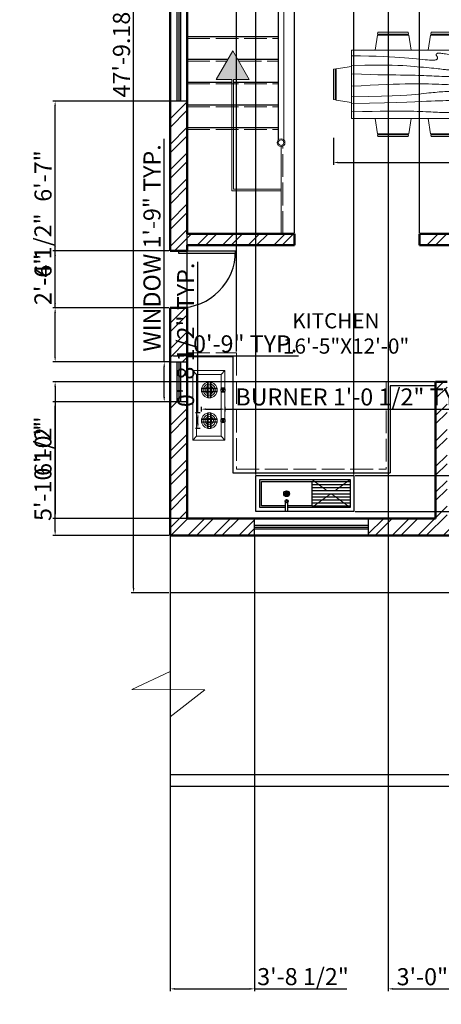
# Model space of a CAD drawing. Units: inches. Extents: x 635 to 1184, y 1837 to 2697.
# Tile 1 of 6: x 635 to 857, y 1837 to 2356. Entities that reach past the tile are written whole.
import ezdxf

# ---------------------------------------------------------------- set-up
doc = ezdxf.new("R2010")
doc.units = ezdxf.units.IN
doc.linetypes.add('ACAD_ISO02W100', pattern=[15, 12, -3])
for name, color, linetype, lineweight in [('A-ANNO-DIMS', 2, 'Continuous', 18), ('A-ANNO-SYMB', 7, 'Continuous', 18), ('A-AREA-IDEN', 7, 'Continuous', 25), ('A-CSWK', 8, 'Continuous', 25), ('A-CSWK-HIDN', 8, 'ACAD_ISO02W100', 13), ('A-DOOR', 4, 'Continuous', 25), ('A-EQPM', 9, 'Continuous', 18), ('A-FLOR-FIXT', 8, 'Continuous', 25), ('A-FLOR-FIXT-HIDN', 8, 'ACAD_ISO02W100', 13), ('A-FLOR-RAIL', 7, 'Continuous', 18), ('A-FLOR-RAIL-HIDN', 8, 'ACAD_ISO02W100', 13), ('A-FLOR-STRS', 7, 'Continuous', 25), ('A-FLOR-STRS-HIDN', 8, 'ACAD_ISO02W100', 13), ('A-FURN', 8, 'Continuous', 18), ('A-GLAZ', 244, 'Continuous', 25), ('A-WALL', 7, 'Continuous', 50), ('A-WALL-PATT', 252, 'Continuous', 13), ('C-ROAD', 8, 'Continuous', 25)]:
    doc.layers.add(name, color=color, linetype=linetype, lineweight=lineweight)
doc.styles.get("Standard").update_dxf_attribs({"font": 'arial.ttf'})
doc.dimstyles.new('ISO-25', dxfattribs={"dimtxt": 9, "dimasz": 2.5, "dimexe": 1.25, "dimexo": 0.625, "dimtad": 1, "dimlunit": 3, "dimtxsty": 'Standard', "dimcen": 2.5, "dimadec": 0, "dimazin": 0, "dimtfac": 1, "dimtmove": 0, "dimatfit": 3, "dimfxl": 1, "dimarcsym": 0})

# ---------------------------------------------------------------- blocks, each defined once
blk = doc.blocks.new('*U5')
for p, q in [((-40, 0), (-40, 6)), ((0, 0), (0, 6))]:
    blk.add_line(p, q)
blk.add_lwpolyline([(0, 0), (0, -40), (-1.75, -40), (-1.75, 0)], close=True)
blk.add_arc((0, 0), 40, 180, 270)
blk = doc.blocks.new('Dining Set - 36 x 72 in.')
for p, q in [((-22.2343, 26.00059), (-23.4847, 17.99762)), ((-22.2304, 26), (-5.7608, 26)), ((-22, 27.5), (-22.1562, 26.50042)), ((-5.8416, 26.5), (-22.1534, 26.5)), ((-22, 27.5), (-6, 27.5)), ((-5.8437, 26.49966), (-6, 27.5)), ((-4.5152, 17.99762), (-5.7655, 25.99926)), ((5.7657, 26.00059), (4.5153, 17.99762)), ((5.7696, 26), (22.2392, 26)), ((6, 27.5), (5.8438, 26.50042)), ((22.1584, 26.5), (5.8466, 26.5)), ((6, 27.5), (22, 27.5)), ((22.1563, 26.49966), (22, 27.5)), ((23.4848, 17.99762), (22.2345, 25.99926)), ((36, 18), (-36, 18)), ((-36, 18), (-36, -18)), ((36, -18), (36, 18)), ((-45.5, 8), (-44.5004, 8.15617)), ((-45.5, 8), (-45.5, -8)), ((-44.5, -8.15843), (-44.5, 8.15338)), ((-44.0006, 8.23428), (-35.9976, 9.48474)), ((-44, 8.23041), (-44, -8.23915)), ((44.0006, 8.23428), (35.9976, 9.48474)), ((44, 8.23041), (44, -8.23915)), ((44.5, -8.15843), (44.5, 8.15338)), ((45.5, 8), (44.5005, 8.15617)), ((45.5, 8), (45.5, -8)), ((-44.4997, -8.15631), (-45.5, -8)), ((-35.9976, -9.48476), (-43.9993, -8.2345)), ((35.9976, -9.48476), (43.9993, -8.2345)), ((44.4997, -8.15631), (45.5, -8)), ((-36, -18), (36, -18)), ((-22.2343, -26.0006), (-23.4847, -17.99762)), ((-4.5152, -17.99762), (-5.7655, -25.99928)), ((5.7657, -26.0006), (4.5153, -17.99762)), ((23.4848, -17.99762), (22.2345, -25.99928)), ((-22.2304, -26), (-5.7608, -26)), ((-22, -27.5), (-22.1562, -26.50044)), ((-5.8416, -26.5), (-22.1534, -26.5)), ((-22, -27.5), (-6, -27.5)), ((-5.8437, -26.49967), (-6, -27.5)), ((5.7696, -26), (22.2392, -26)), ((6, -27.5), (5.8438, -26.50044)), ((22.1584, -26.5), (5.8466, -26.5)), ((6, -27.5), (22, -27.5)), ((22.1563, -26.49967), (22, -27.5))]:
    blk.add_line(p, q)
for points in [[(-36, 15), (-31.1772, 14.97754), (-26.8079, 14.91406), (-22.8538, 14.81543), (-19.276, 14.6875), (-16.0362, 14.53613), (-13.0957, 14.36718), (-10.4159, 14.18652), (-7.9583, 14), (-5.6904, 13.81315), (-3.6035, 13.63021), (-1.6954, 13.45508), (0.0365, 13.29166), (1.5945, 13.14388), (2.9811, 13.01562), (4.1988, 12.9108), (5.25, 12.83333), (6.1393, 12.78613), (6.8802, 12.76823), (7.4883, 12.77767), (7.9792, 12.8125), (8.3685, 12.87077), (8.6719, 12.95052), (8.9049, 13.0498), (9.0833, 13.16666), (9.2205, 13.29899), (9.3216, 13.44401), (9.3895, 13.59879), (9.4271, 13.76041), (9.4373, 13.92594), (9.4232, 14.09245), (9.3875, 14.257), (9.3333, 14.41666), (9.2638, 14.56917), (9.1836, 14.71484), (9.0975, 14.85465), (9.0104, 14.98958), (8.9272, 15.1206), (8.8529, 15.2487), (8.7922, 15.37483), (8.75, 15.5), (8.7305, 15.62467), (8.7344, 15.74739), (8.7617, 15.86621), (8.8125, 15.97916), (8.8867, 16.08431), (8.9844, 16.17968), (9.1055, 16.26334), (9.25, 16.33333), (9.4189, 16.38802), (9.6172, 16.42708), (9.8506, 16.45052), (10.125, 16.45833), (10.4463, 16.45052), (10.8203, 16.42708), (11.2529, 16.38802), (11.75, 16.33333), (12.3184, 16.26318), (12.9694, 16.17838), (13.7151, 16.07991), (14.5677, 15.96875), (15.5395, 15.84586), (16.6426, 15.71224), (17.8893, 15.56884), (19.2917, 15.41666), (20.859, 15.25667), (22.5879, 15.08984), (24.4721, 14.91715), (26.5052, 14.73958), (28.6809, 14.5581), (30.9929, 14.3737), (33.4347, 14.18733), (36, 14)], [(-36, 10), (-28.9766, 10.14274), (-23.1725, 10.20442), (-18.4241, 10.19775), (-14.5677, 10.13541), (-11.4399, 10.03011), (-8.877, 9.89453), (-6.7154, 9.74137), (-4.7917, 9.58333), (-2.9698, 9.43082), (-1.2246, 9.28515), (0.4415, 9.14534), (2.026, 9.01041), (3.5266, 8.87939), (4.9408, 8.7513), (6.266, 8.62516), (7.5, 8.5), (8.6411, 8.37549), (9.6914, 8.2539), (10.6538, 8.13818), (11.5312, 8.03125), (12.3267, 7.93603), (13.043, 7.85547), (13.6831, 7.79248), (14.25, 7.75), (14.7471, 7.7303), (15.1797, 7.73307), (15.5537, 7.75732), (15.875, 7.80208), (16.1494, 7.86637), (16.3828, 7.94922), (16.5811, 8.04964), (16.75, 8.16666), (16.8944, 8.29915), (17.0143, 8.44531), (17.1089, 8.60319), (17.1771, 8.77083), (17.218, 8.94629), (17.2305, 9.1276), (17.2137, 9.31282), (17.1667, 9.5), (17.0895, 9.6875), (16.987, 9.875), (16.8649, 10.0625), (16.7292, 10.25), (16.5856, 10.4375), (16.4401, 10.625), (16.2985, 10.8125), (16.1667, 11), (16.05, 11.18733), (15.9518, 11.3737), (15.8752, 11.5581), (15.8229, 11.73958), (15.798, 11.91715), (15.8034, 12.08984), (15.842, 12.25667), (15.9167, 12.41666), (16.0295, 12.56836), (16.1784, 12.70833), (16.3605, 12.83268), (16.5729, 12.9375), (16.8127, 13.01888), (17.0768, 13.07291), (17.3625, 13.0957), (17.6667, 13.08333), (17.9894, 13.03312), (18.3418, 12.94726), (18.7382, 12.82918), (19.1927, 12.68229), (19.7195, 12.51001), (20.3327, 12.31575), (21.0465, 12.10294), (21.875, 11.875), (22.8357, 11.63354), (23.959, 11.37304), (25.2786, 11.08618), (26.8282, 10.76562), (28.6414, 10.40405), (30.752, 9.99414), (33.1936, 9.52856), (36, 9)], [(-36, 5.5), (-30.7157, 5.3348), (-26.069, 5.20963), (-21.9946, 5.11767), (-18.4271, 5.05208), (-15.3009, 5.00602), (-12.5508, 4.97265), (-10.1112, 4.94515), (-7.9167, 4.91666), (-5.909, 4.88167), (-4.0586, 4.83984), (-2.3429, 4.79215), (-0.7396, 4.73958), (0.7739, 4.6831), (2.22, 4.6237), (3.6213, 4.56233), (5, 4.5), (6.373, 4.43782), (7.7344, 4.3776), (9.0723, 4.32129), (10.375, 4.27083), (11.6309, 4.22819), (12.8281, 4.19531), (13.9551, 4.17415), (15, 4.16666), (15.954, 4.17448), (16.819, 4.19791), (17.6001, 4.23698), (18.3021, 4.29166), (18.9299, 4.36198), (19.4883, 4.44791), (19.9823, 4.54948), (20.4167, 4.66666), (20.7969, 4.79899), (21.1302, 4.94401), (21.4245, 5.09879), (21.6875, 5.26041), (21.9271, 5.42594), (22.1511, 5.59245), (22.3672, 5.757), (22.5834, 5.91666), (22.8065, 6.06868), (23.0404, 6.21093), (23.2879, 6.34147), (23.5521, 6.45833), (23.8358, 6.55957), (24.142, 6.64323), (24.4735, 6.70735), (24.8334, 6.75), (25.2235, 6.76969), (25.642, 6.76692), (26.0858, 6.74267), (26.5521, 6.69791), (27.0379, 6.63362), (27.5404, 6.55078), (28.0565, 6.45036), (28.5834, 6.33333), (29.1242, 6.19987), (29.7071, 6.04687), (30.3661, 5.87044), (31.1354, 5.66666), (32.0493, 5.43164), (33.142, 5.16146), (34.4475, 4.85221), (36, 4.5)], [(-36, -1), (-30.7915, -0.6591), (-26.0195, -0.38216), (-21.6519, -0.16284), (-17.6563, 0.00521), (-14.0005, 0.12833), (-10.6523, 0.21289), (-7.5796, 0.26522), (-4.75, 0.29166), (-2.134, 0.29793), (0.2878, 0.28711), (2.5317, 0.26163), (4.6146, 0.22396), (6.5529, 0.17651), (8.3633, 0.12174), (10.0623, 0.06209), (11.6667, 0), (13.1899, -0.06201), (14.6341, -0.1211), (15.9982, -0.17432), (17.2813, -0.21875), (18.4823, -0.25147), (19.6003, -0.26953), (20.6343, -0.27002), (21.5834, -0.25), (22.4481, -0.20768), (23.2357, -0.14584), (23.9549, -0.06836), (24.6146, 0.02083), (25.2235, 0.11784), (25.7904, 0.21875), (26.3241, 0.31966), (26.8334, 0.41666), (27.3265, 0.50618), (27.8099, 0.58593), (28.2894, 0.65397), (28.7709, 0.70833), (29.2601, 0.74707), (29.763, 0.76823), (30.2855, 0.76985), (30.8334, 0.75), (31.4088, 0.70784), (31.9994, 0.64713), (32.589, 0.57275), (33.1615, 0.48958), (33.7008, 0.4025), (34.1908, 0.3164), (34.6153, 0.23616), (34.9584, 0.16666), (35.2099, 0.11165), (35.3848, 0.07031), (35.504, 0.04069), (35.5886, 0.02083), (35.6594, 0.00879), (35.7377, 0.0026), (35.8442, 0.00032), (36, 0)], [(-36, -6.5), (-27.1843, -6.31267), (-20.084, -6.1263), (-14.469, -5.9419), (-10.1094, -5.76042), (-6.7752, -5.58285), (-4.2363, -5.41016), (-2.2629, -5.24333), (-0.625, -5.08334), (0.8708, -4.93099), (2.2715, -4.78646), (3.5872, -4.64974), (4.8281, -4.52084), (6.0046, -4.39974), (7.127, -4.28646), (8.2053, -4.18099), (9.25, -4.08334), (10.2705, -3.99382), (11.2734, -3.91407), (12.2647, -3.84603), (13.25, -3.79167), (14.2354, -3.75293), (15.2266, -3.73177), (16.2295, -3.73015), (17.25, -3.75), (18.2912, -3.79248), (19.3451, -3.85547), (20.4009, -3.93604), (21.4479, -4.03125), (22.4754, -4.13819), (23.4727, -4.25391), (24.4289, -4.37549), (25.3334, -4.5), (26.1785, -4.62492), (26.9694, -4.74935), (27.7145, -4.87281), (28.4219, -4.99479), (29.1, -5.11483), (29.7572, -5.23242), (30.4016, -5.34709), (31.0417, -5.45834), (31.6837, -5.56437), (32.3262, -5.65821), (32.9658, -5.73153), (33.599, -5.77604), (34.2224, -5.78345), (34.8327, -5.74545), (35.4264, -5.65373), (36, -5.5)], [(-36, -10), (-26.4022, -9.81299), (-18.4675, -9.62891), (-11.9839, -9.45069), (-6.7396, -9.28125), (-2.5226, -9.12354), (0.8789, -8.98047), (3.6769, -8.85498), (6.0833, -8.75), (8.2767, -8.66765), (10.3021, -8.60677), (12.1712, -8.56543), (13.8958, -8.54167), (15.4876, -8.53353), (16.9583, -8.53907), (18.3197, -8.55632), (19.5834, -8.58334), (20.7616, -8.61841), (21.8685, -8.66081), (22.9188, -8.71004), (23.9271, -8.76563), (24.9081, -8.82707), (25.8763, -8.89388), (26.8465, -8.96558), (27.8334, -9.04167), (28.8474, -9.12118), (29.8828, -9.20117), (30.93, -9.27824), (31.9792, -9.34896), (33.0205, -9.40991), (34.0443, -9.45768), (35.0407, -9.48885), (36, -9.5)], [(-36, -14.5), (-30.0881, -14.33513), (-25.0332, -14.21224), (-20.7312, -14.12647), (-17.0781, -14.07292), (-13.97, -14.04671), (-11.3027, -14.04297), (-8.9724, -14.05681), (-6.875, -14.08334), (-4.9224, -14.11833), (-3.0905, -14.16016), (-1.3709, -14.20785), (0.2448, -14.26042), (1.7647, -14.3169), (3.1973, -14.3763), (4.5507, -14.43767), (5.8333, -14.5), (7.0554, -14.5621), (8.235, -14.62175), (9.3922, -14.67652), (10.5469, -14.72396), (11.7192, -14.76164), (12.929, -14.78711), (14.1965, -14.79794), (15.5417, -14.79167), (16.9933, -14.76424), (18.6152, -14.70508), (20.4804, -14.60197), (22.6615, -14.44271), (25.2312, -14.21509), (28.2624, -13.9069), (31.8277, -13.50594), (36, -13)]]:
    blk.add_lwpolyline(points)
blk = doc.blocks.new('*D17')
at = {"layer": 'A-ANNO-DIMS', "color": 0, "lineweight": -2, "transparency": 16777216}
for p, q in [((713.66, 2627.14), (693.72, 2627.14)), ((694.97, 2056.46), (694.97, 2624.64)), ((713.66, 2053.96), (693.72, 2053.96))]:
    blk.add_line(p, q, dxfattribs=at)
at = {"layer": 'A-ANNO-DIMS', "color": 0, "transparency": 16777216}
for points in [[(694.56, 2624.64), (695.39, 2624.64), (694.97, 2627.14)], [(694.56, 2056.46), (695.39, 2056.46), (694.97, 2053.96)]]:
    blk.add_solid(points, dxfattribs=at)
at = {"layer": 'DEFPOINTS', "color": 0, "transparency": 16777216}
for p in [(694.97, 2627.14), (714.28, 2627.14), (714.28, 2053.96)]:
    blk.add_point(p, dxfattribs=at)
at = {"layer": 'A-ANNO-DIMS', "color": 0, "transparency": 16777216, "insert": (689.75, 2340.55), "char_height": 9, "attachment_point": 5, "rotation": 90}
blk.add_mtext('47\'-9.18"', dxfattribs=at)
blk = doc.blocks.new('WIN-21IN')
for p, q in [((3.5, 21), (3.5, 0)), ((4.5, 21), (4.5, 0)), ((5.5, 21), (5.5, 0))]:
    blk.add_line(p, q)
blk.add_lwpolyline([(0, 21), (9, 21), (9, 0), (0, 0)], close=True)
blk = doc.blocks.new('WIN-60IN')
for p, q in [((0, 5.5), (60, 5.5)), ((0, 4.5), (60, 4.5)), ((0, 3.5), (60, 3.5))]:
    blk.add_line(p, q)
blk.add_lwpolyline([(0, 9), (60, 9), (60, 0), (0, 0)], close=True)
blk = doc.blocks.new('COOKTOP-BURNER-WITH-CONTROL')
for p, q in [((3.26, 8.21), (3.26, 0.1)), ((3.56, 8.27), (3.56, 5.06)), ((4.76, 8.27), (4.76, 5.06)), ((5.06, 8.21), (5.06, 0.1)), ((11.16, 5.31), (11.16, 3)), ((11.56, 5.31), (11.56, 3)), ((0.04, 4.76), (3.26, 4.76)), ((0.04, 3.56), (3.26, 3.56)), ((0.1, 5.06), (8.21, 5.06)), ((0.1, 3.26), (8.21, 3.26)), ((3.56, 4.76), (3.56, 3.56)), ((3.56, 4.76), (4.76, 4.76)), ((3.56, 3.56), (4.76, 3.56)), ((3.56, 3.26), (3.56, 0.04)), ((4.76, 4.76), (4.76, 3.56)), ((4.76, 3.26), (4.76, 0.04)), ((5.06, 4.76), (8.27, 4.76)), ((5.06, 3.56), (8.27, 3.56))]:
    blk.add_line(p, q)
for centre, radius in [((4.16, 4.16), 4.16), ((11.36, 4.16), 1.17)]:
    blk.add_circle(centre, radius)
for centre, radius, start, end in [((4.16, 4.16), 3.16, 106.5657, 163.4343), ((4.16, 4.16), 2.16, 114.6654, 155.3346), ((4.16, 4.16), 1.16, 51.0893, 128.9107), ((4.16, 4.16), 3.16, 79.0428, 100.9572), ((4.16, 4.16), 2.16, 73.8464, 106.1536), ((4.16, 4.16), 3.16, 16.5657, 73.4343), ((4.16, 4.16), 2.16, 24.6654, 65.3346), ((4.16, 4.16), 3.16, 169.0428, 190.9572), ((4.16, 4.16), 3.16, 196.5657, 253.4343), ((4.16, 4.16), 2.16, 163.8464, 196.1536), ((4.16, 4.16), 2.16, 204.6654, 245.3346), ((4.16, 4.16), 1.16, 141.0893, 218.9107), ((4.16, 4.16), 1.16, 231.0893, 308.9107), ((4.16, 4.16), 2.16, 253.8464, 286.1536), ((4.16, 4.16), 3.16, 259.0428, 280.9572), ((4.16, 4.16), 1.16, 321.0893, 38.9107), ((4.16, 4.16), 2.16, 294.6654, 335.3346), ((4.16, 4.16), 3.16, 286.5657, 343.4343), ((4.16, 4.16), 2.16, 343.8464, 16.1536), ((4.16, 4.16), 3.16, 349.0428, 10.9572), ((11.36, 4.16), 0.574, 110.3869, 249.6131), ((11.36, 4.16), 0.574, 290.3869, 69.6131)]:
    blk.add_arc(centre, radius, start, end)
blk = doc.blocks.new('*D25')
at = {"layer": 'A-ANNO-DIMS', "color": 0, "lineweight": -2, "transparency": 16777216}
for p, q in [((711.13, 2175.64), (711.13, 2293.28)), ((713.66, 2175.64), (709.88, 2175.64)), ((711.13, 2157.14), (711.13, 2173.14)), ((713.66, 2154.64), (709.88, 2154.64))]:
    blk.add_line(p, q, dxfattribs=at)
at = {"layer": 'A-ANNO-DIMS', "color": 0, "transparency": 16777216}
for points in [[(710.72, 2173.14), (711.55, 2173.14), (711.13, 2175.64)], [(710.72, 2157.14), (711.55, 2157.14), (711.13, 2154.64)]]:
    blk.add_solid(points, dxfattribs=at)
at = {"layer": 'DEFPOINTS', "color": 0, "transparency": 16777216}
for p in [(711.13, 2175.64), (714.28, 2175.64), (714.28, 2154.64)]:
    blk.add_point(p, dxfattribs=at)
at = {"layer": 'A-ANNO-DIMS', "color": 0, "transparency": 16777216, "insert": (705.85, 2235.71), "char_height": 9, "attachment_point": 5, "rotation": 90}
blk.add_mtext('WINDOW 1\'-9" TYP.', dxfattribs=at)
blk = doc.blocks.new('*D26')
at = {"layer": 'A-ANNO-DIMS', "color": 0, "lineweight": -2, "transparency": 16777216}
for p, q in [((714.28, 2176.27), (714.28, 2180.04)), ((723.28, 2176.27), (723.28, 2180.04)), ((716.78, 2178.79), (720.78, 2178.79)), ((723.28, 2178.79), (781.89, 2178.79))]:
    blk.add_line(p, q, dxfattribs=at)
at = {"layer": 'A-ANNO-DIMS', "color": 0, "transparency": 16777216}
for points in [[(716.78, 2179.21), (716.78, 2178.38), (714.28, 2178.79)], [(720.78, 2179.21), (720.78, 2178.38), (723.28, 2178.79)]]:
    blk.add_solid(points, dxfattribs=at)
at = {"layer": 'DEFPOINTS', "color": 0, "transparency": 16777216}
for p in [(714.28, 2175.64), (723.28, 2178.79), (723.28, 2175.64)]:
    blk.add_point(p, dxfattribs=at)
at = {"layer": 'A-ANNO-DIMS', "color": 0, "transparency": 16777216, "insert": (753.84, 2184.01), "char_height": 9, "attachment_point": 5}
blk.add_mtext('0\'-9" TYP.', dxfattribs=at)
blk = doc.blocks.new('*D31')
at = {"layer": 'A-ANNO-DIMS', "color": 0, "lineweight": -2, "transparency": 16777216}
for p, q in [((730.76, 2149.5), (730.76, 2152.01)), ((733.26, 2150.76), (740.79, 2150.76)), ((743.29, 2149.5), (743.29, 2152.01)), ((743.29, 2150.76), (879.06, 2150.76))]:
    blk.add_line(p, q, dxfattribs=at)
at = {"layer": 'A-ANNO-DIMS', "color": 0, "transparency": 16777216}
for points in [[(733.26, 2151.18), (733.26, 2150.34), (730.76, 2150.76)], [(740.79, 2151.18), (740.79, 2150.34), (743.29, 2150.76)]]:
    blk.add_solid(points, dxfattribs=at)
at = {"layer": 'DEFPOINTS', "color": 0, "transparency": 16777216}
for p in [(730.76, 2148.88), (743.29, 2150.76), (743.29, 2148.88)]:
    blk.add_point(p, dxfattribs=at)
at = {"layer": 'A-ANNO-DIMS', "color": 0, "transparency": 16777216, "insert": (812.43, 2156.04), "char_height": 9, "attachment_point": 5}
blk.add_mtext('BURNER 1\'-0 1/2" TYP.', dxfattribs=at)
blk = doc.blocks.new('*D32')
at = {"layer": 'A-ANNO-DIMS', "color": 0, "lineweight": -2, "transparency": 16777216}
for p, q in [((728.88, 2148.88), (728.88, 2228.46)), ((730.14, 2148.88), (727.63, 2148.88)), ((728.88, 2143.07), (728.88, 2146.38)), ((730.14, 2140.57), (727.63, 2140.57))]:
    blk.add_line(p, q, dxfattribs=at)
at = {"layer": 'A-ANNO-DIMS', "color": 0, "transparency": 16777216}
for points in [[(728.46, 2146.38), (729.3, 2146.38), (728.88, 2148.88)], [(728.46, 2143.07), (729.3, 2143.07), (728.88, 2140.57)]]:
    blk.add_solid(points, dxfattribs=at)
at = {"layer": 'DEFPOINTS', "color": 0, "transparency": 16777216}
for p in [(728.88, 2148.88), (730.76, 2148.88), (730.76, 2140.57)]:
    blk.add_point(p, dxfattribs=at)
at = {"layer": 'A-ANNO-DIMS', "color": 0, "transparency": 16777216, "insert": (723.6, 2189.92), "char_height": 9, "attachment_point": 5, "rotation": 90}
blk.add_mtext('0\'-8 1/2" TYP.', dxfattribs=at)
blk = doc.blocks.new('*D37')
at = {"layer": 'A-ANNO-DIMS', "color": 0, "lineweight": -2, "transparency": 16777216}
for p, q in [((800.35, 2293.79), (800.35, 2279.52)), ((891.35, 2293.79), (891.35, 2279.52)), ((802.85, 2280.77), (888.85, 2280.77)), ((891.35, 2280.77), (994.02, 2280.77))]:
    blk.add_line(p, q, dxfattribs=at)
at = {"layer": 'A-ANNO-DIMS', "color": 0, "transparency": 16777216}
for points in [[(802.85, 2281.18), (802.85, 2280.35), (800.35, 2280.77)], [(888.85, 2281.18), (888.85, 2280.35), (891.35, 2280.77)]]:
    blk.add_solid(points, dxfattribs=at)
at = {"layer": 'DEFPOINTS', "color": 0, "transparency": 16777216}
for p in [(800.35, 2294.42), (891.35, 2294.42), (891.35, 2280.77)]:
    blk.add_point(p, dxfattribs=at)
at = {"layer": 'A-ANNO-DIMS', "color": 0, "transparency": 16777216, "insert": (943.93, 2286.05), "char_height": 9, "attachment_point": 5}
blk.add_mtext('DINING SET 7\'-7"', dxfattribs=at)
blk = doc.blocks.new('*D41')
at = {"layer": 'A-ANNO-DIMS', "color": 0, "lineweight": -2, "transparency": 16777216}
for p, q in [((713.66, 2313.14), (652.36, 2313.14)), ((653.61, 2236.64), (653.61, 2310.64)), ((713.66, 2234.14), (652.36, 2234.14))]:
    blk.add_line(p, q, dxfattribs=at)
at = {"layer": 'A-ANNO-DIMS', "color": 0, "transparency": 16777216}
for points in [[(653.2, 2310.64), (654.03, 2310.64), (653.61, 2313.14)], [(653.2, 2236.64), (654.03, 2236.64), (653.61, 2234.14)]]:
    blk.add_solid(points, dxfattribs=at)
at = {"layer": 'DEFPOINTS', "color": 0, "transparency": 16777216}
for p in [(653.61, 2313.14), (714.28, 2313.14), (714.28, 2234.14)]:
    blk.add_point(p, dxfattribs=at)
at = {"layer": 'A-ANNO-DIMS', "color": 0, "transparency": 16777216, "insert": (648.39, 2273.64), "char_height": 9, "attachment_point": 5, "rotation": 90}
blk.add_mtext('6\'-7"', dxfattribs=at)
blk = doc.blocks.new('*D46')
at = {"layer": 'A-ANNO-DIMS', "color": 0, "lineweight": -2, "transparency": 16777216}
for p, q in [((713.66, 2234.14), (652.36, 2234.14)), ((653.61, 2206.64), (653.61, 2231.64)), ((713.66, 2204.14), (652.36, 2204.14))]:
    blk.add_line(p, q, dxfattribs=at)
at = {"layer": 'A-ANNO-DIMS', "color": 0, "transparency": 16777216}
for points in [[(653.2, 2231.64), (654.03, 2231.64), (653.61, 2234.14)], [(653.2, 2206.64), (654.03, 2206.64), (653.61, 2204.14)]]:
    blk.add_solid(points, dxfattribs=at)
at = {"layer": 'DEFPOINTS', "color": 0, "transparency": 16777216}
for p in [(653.61, 2234.14), (714.28, 2234.14), (714.28, 2204.14)]:
    blk.add_point(p, dxfattribs=at)
at = {"layer": 'A-ANNO-DIMS', "color": 0, "transparency": 16777216, "insert": (648.39, 2219.14), "char_height": 9, "attachment_point": 5, "rotation": 90}
blk.add_mtext('2\'-6"', dxfattribs=at)
blk = doc.blocks.new('*D47')
at = {"layer": 'A-ANNO-DIMS', "color": 0, "lineweight": -2, "transparency": 16777216}
for p, q in [((713.66, 2154.64), (652.36, 2154.64)), ((653.61, 2086.64), (653.61, 2152.14)), ((713.66, 2084.14), (652.36, 2084.14))]:
    blk.add_line(p, q, dxfattribs=at)
at = {"layer": 'A-ANNO-DIMS', "color": 0, "transparency": 16777216}
for points in [[(653.2, 2152.14), (654.03, 2152.14), (653.61, 2154.64)], [(653.2, 2086.64), (654.03, 2086.64), (653.61, 2084.14)]]:
    blk.add_solid(points, dxfattribs=at)
at = {"layer": 'DEFPOINTS', "color": 0, "transparency": 16777216}
for p in [(653.61, 2154.64), (714.28, 2154.64), (714.28, 2084.14)]:
    blk.add_point(p, dxfattribs=at)
at = {"layer": 'A-ANNO-DIMS', "color": 0, "transparency": 16777216, "insert": (648.34, 2119.39), "char_height": 9, "attachment_point": 5, "rotation": 90}
blk.add_mtext('5\'-10 1/2"', dxfattribs=at)
blk = doc.blocks.new('*D48')
at = {"layer": 'A-ANNO-DIMS', "color": 0, "lineweight": -2, "transparency": 16777216}
for p, q in [((653.61, 2204.14), (653.61, 2252.94)), ((713.66, 2204.14), (652.36, 2204.14)), ((653.61, 2178.14), (653.61, 2201.64)), ((713.66, 2175.64), (652.36, 2175.64))]:
    blk.add_line(p, q, dxfattribs=at)
at = {"layer": 'A-ANNO-DIMS', "color": 0, "transparency": 16777216}
for points in [[(653.2, 2201.64), (654.03, 2201.64), (653.61, 2204.14)], [(653.2, 2178.14), (654.03, 2178.14), (653.61, 2175.64)]]:
    blk.add_solid(points, dxfattribs=at)
at = {"layer": 'DEFPOINTS', "color": 0, "transparency": 16777216}
for p in [(653.61, 2204.14), (714.28, 2204.14), (714.28, 2175.64)]:
    blk.add_point(p, dxfattribs=at)
at = {"layer": 'A-ANNO-DIMS', "color": 0, "transparency": 16777216, "insert": (648.34, 2229.79), "char_height": 9, "attachment_point": 5, "rotation": 90}
blk.add_mtext('2\'-4 1/2"', dxfattribs=at)
blk = doc.blocks.new('*D56')
at = {"layer": 'A-ANNO-DIMS', "color": 0, "lineweight": -2, "transparency": 16777216}
for p, q in [((759.51, 2116.34), (759.51, 2668.89)), ((762.01, 2667.64), (808.65, 2667.64)), ((811.15, 2116.34), (811.15, 2668.89))]:
    blk.add_line(p, q, dxfattribs=at)
at = {"layer": 'A-ANNO-DIMS', "color": 0, "transparency": 16777216}
for points in [[(762.01, 2668.06), (762.01, 2667.23), (759.51, 2667.64)], [(808.65, 2668.06), (808.65, 2667.23), (811.15, 2667.64)]]:
    blk.add_solid(points, dxfattribs=at)
at = {"layer": 'DEFPOINTS', "color": 0, "transparency": 16777216}
for p in [(811.15, 2667.64), (759.51, 2115.72), (811.15, 2115.72)]:
    blk.add_point(p, dxfattribs=at)
at = {"layer": 'A-ANNO-DIMS', "color": 0, "transparency": 16777216, "insert": (785.33, 2672.92), "char_height": 9, "attachment_point": 5}
blk.add_mtext('4\'-3 1/2"', dxfattribs=at)
blk = doc.blocks.new('*D57')
at = {"layer": 'A-ANNO-DIMS', "color": 0, "lineweight": -2, "transparency": 16777216}
for p, q in [((811.77, 2115.72), (1176.99, 2115.72)), ((1175.74, 2113.22), (1175.74, 2099.39)), ((811.77, 2096.89), (1176.99, 2096.89)), ((1175.74, 2096.89), (1175.74, 2070.06))]:
    blk.add_line(p, q, dxfattribs=at)
at = {"layer": 'A-ANNO-DIMS', "color": 0, "transparency": 16777216}
for points in [[(1175.32, 2113.22), (1176.15, 2113.22), (1175.74, 2115.72)], [(1175.32, 2099.39), (1176.15, 2099.39), (1175.74, 2096.89)]]:
    blk.add_solid(points, dxfattribs=at)
at = {"layer": 'DEFPOINTS', "color": 0, "transparency": 16777216}
for p in [(811.15, 2115.72), (811.15, 2096.89), (1175.74, 2096.89)]:
    blk.add_point(p, dxfattribs=at)
at = {"layer": 'A-ANNO-DIMS', "color": 0, "transparency": 16777216, "insert": (1170.59, 2082.22), "char_height": 9, "attachment_point": 5, "rotation": 90}
blk.add_mtext('1\'-7"', dxfattribs=at)
blk = doc.blocks.new('*D58')
at = {"layer": 'A-ANNO-DIMS', "color": 0, "lineweight": -2, "transparency": 16777216}
for p, q in [((853.66, 2165.14), (652.36, 2165.14)), ((653.61, 2162.64), (653.61, 2095.64)), ((853.66, 2093.14), (652.36, 2093.14))]:
    blk.add_line(p, q, dxfattribs=at)
at = {"layer": 'A-ANNO-DIMS', "color": 0, "transparency": 16777216}
for points in [[(653.2, 2162.64), (654.03, 2162.64), (653.61, 2165.14)], [(653.2, 2095.64), (654.03, 2095.64), (653.61, 2093.14)]]:
    blk.add_solid(points, dxfattribs=at)
at = {"layer": 'DEFPOINTS', "color": 0, "transparency": 16777216}
for p in [(854.28, 2165.14), (653.61, 2093.14), (854.28, 2093.14)]:
    blk.add_point(p, dxfattribs=at)
at = {"layer": 'A-ANNO-DIMS', "color": 0, "transparency": 16777216, "insert": (648.39, 2129.14), "char_height": 9, "attachment_point": 5, "rotation": 90}
blk.add_mtext('6\'-0"', dxfattribs=at)
blk = doc.blocks.new('*D59')
at = {"layer": 'A-ANNO-DIMS', "color": 0, "lineweight": -2, "transparency": 16777216}
for p, q in [((723.28, 2181.16), (723.28, 2668.89)), ((725.78, 2667.64), (746.78, 2667.64)), ((749.28, 2181.16), (749.28, 2668.89))]:
    blk.add_line(p, q, dxfattribs=at)
at = {"layer": 'A-ANNO-DIMS', "color": 0, "transparency": 16777216}
for points in [[(725.78, 2668.06), (725.78, 2667.23), (723.28, 2667.64)], [(746.78, 2668.06), (746.78, 2667.23), (749.28, 2667.64)]]:
    blk.add_solid(points, dxfattribs=at)
at = {"layer": 'DEFPOINTS', "color": 0, "transparency": 16777216}
for p in [(749.28, 2667.64), (723.28, 2180.53), (749.28, 2180.53)]:
    blk.add_point(p, dxfattribs=at)
at = {"layer": 'A-ANNO-DIMS', "color": 0, "transparency": 16777216, "insert": (736.28, 2672.79), "char_height": 9, "attachment_point": 5}
blk.add_mtext('2\'-2"', dxfattribs=at)
blk = doc.blocks.new('*D60')
at = {"layer": 'A-ANNO-DIMS', "color": 0, "lineweight": -2, "transparency": 16777216}
for p, q in [((779.78, 2243.77), (779.78, 2668.89)), ((782.28, 2667.64), (843.28, 2667.64)), ((845.78, 2243.77), (845.78, 2668.89))]:
    blk.add_line(p, q, dxfattribs=at)
at = {"layer": 'A-ANNO-DIMS', "color": 0, "transparency": 16777216}
for points in [[(782.28, 2668.06), (782.28, 2667.23), (779.78, 2667.64)], [(843.28, 2668.06), (843.28, 2667.23), (845.78, 2667.64)]]:
    blk.add_solid(points, dxfattribs=at)
at = {"layer": 'DEFPOINTS', "color": 0, "transparency": 16777216}
for p in [(845.78, 2667.64), (779.78, 2243.14), (845.78, 2243.14)]:
    blk.add_point(p, dxfattribs=at)
at = {"layer": 'A-ANNO-DIMS', "color": 0, "transparency": 16777216, "insert": (812.78, 2672.86), "char_height": 9, "attachment_point": 5}
blk.add_mtext('5\'-6"', dxfattribs=at)
blk = doc.blocks.new('*D61')
at = {"layer": 'A-ANNO-DIMS', "color": 0, "lineweight": -2, "transparency": 16777216}
for p, q in [((714.28, 2083.52), (714.28, 1843.99)), ((758.78, 2083.52), (758.78, 1843.99)), ((716.78, 1845.24), (756.28, 1845.24)), ((758.78, 1845.24), (807.42, 1845.24))]:
    blk.add_line(p, q, dxfattribs=at)
at = {"layer": 'A-ANNO-DIMS', "color": 0, "transparency": 16777216}
for points in [[(716.78, 1845.65), (716.78, 1844.82), (714.28, 1845.24)], [(756.28, 1845.65), (756.28, 1844.82), (758.78, 1845.24)]]:
    blk.add_solid(points, dxfattribs=at)
at = {"layer": 'DEFPOINTS', "color": 0, "transparency": 16777216}
for p in [(714.28, 2084.14), (758.78, 2084.14), (758.78, 1845.24)]:
    blk.add_point(p, dxfattribs=at)
at = {"layer": 'A-ANNO-DIMS', "color": 0, "transparency": 16777216, "insert": (784.35, 1850.52), "char_height": 9, "attachment_point": 5}
blk.add_mtext('3\'-8 1/2"', dxfattribs=at)
blk = doc.blocks.new('*D62')
at = {"layer": 'A-ANNO-DIMS', "color": 0, "lineweight": -2, "transparency": 16777216}
for p, q in [((829.28, 2442.52), (829.28, 1843.99)), ((865.28, 2442.52), (865.28, 1843.99)), ((831.78, 1845.24), (862.78, 1845.24))]:
    blk.add_line(p, q, dxfattribs=at)
at = {"layer": 'A-ANNO-DIMS', "color": 0, "transparency": 16777216}
for points in [[(831.78, 1845.65), (831.78, 1844.82), (829.28, 1845.24)], [(862.78, 1845.65), (862.78, 1844.82), (865.28, 1845.24)]]:
    blk.add_solid(points, dxfattribs=at)
at = {"layer": 'DEFPOINTS', "color": 0, "transparency": 16777216}
for p in [(829.28, 2443.14), (865.28, 2443.14), (865.28, 1845.24)]:
    blk.add_point(p, dxfattribs=at)
at = {"layer": 'A-ANNO-DIMS', "color": 0, "transparency": 16777216, "insert": (847.28, 1850.46), "char_height": 9, "attachment_point": 5}
blk.add_mtext('3\'-0"', dxfattribs=at)

msp = doc.modelspace()

# ---------------------------------------------------------------- hatches: boundary and pattern name
at = {"layer": 'A-ANNO-SYMB'}
h = msp.add_hatch(color=256, dxfattribs=at)
h.dxf.hatch_style = 1
h.paths.add_polyline_path([(978.007, 1908.412), (964.784, 1885.737), (990.387, 1885.737)])
h.paths.add_polyline_path([(747.282, 2339.586), (738.604, 2324.556), (746.882, 2324.556), (746.882, 2322.142), (747.682, 2322.142), (747.682, 2324.556), (755.96, 2324.556)])
at = {"layer": 'A-WALL-PATT'}
h = msp.add_hatch(dxfattribs=at)
h.set_pattern_fill('ANSI32', color=256)
h.paths.add_polyline_path([(723.282, 2313.142), (714.282, 2313.142), (714.282, 2234.142), (718.782, 2234.142), (723.282, 2234.142), (723.282, 2237.142), (779.782, 2237.142), (779.782, 2243.142), (723.282, 2243.142)])
h.paths.add_polyline_path([(926.282, 2320.142), (920.282, 2320.142), (920.282, 2243.142), (845.782, 2243.142), (845.782, 2237.142), (920.282, 2237.142), (920.282, 2093.142), (860.282, 2093.142), (860.282, 2165.142), (854.282, 2165.142), (854.282, 2093.142), (818.782, 2093.142), (818.782, 2084.142), (929.282, 2084.142), (929.282, 2156.142), (932.282, 2156.142), (932.282, 2165.142), (926.282, 2165.142)])
h.paths.add_polyline_path([(1075.282, 2250.443), (1066.282, 2250.443), (1066.282, 2233.442), (1075.282, 2233.442)])
h.paths.add_polyline_path([(1075.282, 2173.442), (1066.282, 2173.442), (1066.282, 2165.142), (1057.782, 2165.142), (1057.782, 2156.142), (1075.282, 2156.142)])
h.paths.add_polyline_path([(997.782, 2165.142), (980.282, 2165.142), (980.282, 2156.142), (997.782, 2156.142)])
h.paths.add_polyline_path([(1075.282, 2338.142), (1066.282, 2338.142), (1066.282, 2310.443), (1075.282, 2310.443)])
h.paths.add_polyline_path([(758.782, 2093.142), (723.282, 2093.142), (723.282, 2154.642), (714.282, 2154.642), (714.282, 2084.142), (758.782, 2084.142)])
h.paths.add_polyline_path([(723.282, 2204.142), (714.282, 2204.142), (714.282, 2175.642), (723.282, 2175.642)])
h.paths.add_polyline_path([(1075.282, 2404.069), (1066.282, 2404.069), (1066.282, 2383.142), (970.282, 2383.142), (970.282, 2386.142), (964.282, 2386.142), (964.282, 2383.142), (926.282, 2383.142), (926.282, 2389.142), (920.282, 2389.142), (920.282, 2368.142), (926.282, 2368.142), (926.282, 2377.142), (1066.282, 2377.142), (1066.282, 2374.142), (1075.282, 2374.142)])
h.paths.add_polyline_path([(926.282, 2443.142), (964.282, 2443.142), (964.282, 2416.142), (970.282, 2416.142), (970.282, 2443.142), (1066.282, 2443.142), (1066.282, 2425.069), (1075.282, 2425.069), (1075.282, 2503.642), (1066.282, 2503.642), (1066.282, 2449.142), (865.282, 2449.142), (865.282, 2443.142), (920.282, 2443.142), (920.282, 2416.142), (926.282, 2416.142)])
h.paths.add_polyline_path([(829.282, 2449.142), (826.282, 2449.142), (826.282, 2527.142), (826.282, 2557.642), (820.282, 2557.642), (820.282, 2527.142), (817.282, 2527.142), (817.282, 2521.142), (820.282, 2521.142), (820.282, 2449.142), (723.282, 2449.142), (723.282, 2474.642), (714.282, 2474.642), (714.282, 2373.142), (723.282, 2373.142), (723.282, 2443.142), (829.282, 2443.142)])
h.paths.add_polyline_path([(787.282, 2527.142), (723.282, 2527.142), (723.282, 2618.142), (820.282, 2618.142), (820.282, 2587.642), (826.282, 2587.642), (826.282, 2618.142), (916.282, 2618.142), (916.282, 2627.142), (714.282, 2627.142), (714.282, 2495.642), (723.282, 2495.642), (723.282, 2521.142), (787.282, 2521.142)])
h.paths.add_polyline_path([(1075.282, 2627.142), (976.282, 2627.142), (976.282, 2618.142), (1066.282, 2618.142), (1066.282, 2563.642), (1075.282, 2563.642)])

# ---------------------------------------------------------------- linework, layer by layer
at = {"layer": 'A-ANNO-SYMB'}
for p, q in [((746.882, 2324.556), (746.882, 2265.889)), ((747.682, 2324.556), (747.682, 2266.689)), ((772.782, 2265.889), (746.882, 2265.889)), ((772.782, 2266.689), (747.682, 2266.689))]:
    msp.add_line(p, q, dxfattribs=at)
for points in [[(747.682, 2324.556), (755.96, 2324.556), (747.282, 2339.586), (738.604, 2324.556), (746.882, 2324.556)], [(714.366, 2055.625), (714.366, 2012.552), (694.114, 2003.087), (732.57, 2002.837), (714.366, 1988.567), (714.366, 1950.712)]]:
    msp.add_lwpolyline(points, dxfattribs=at)
at = {"layer": 'A-CSWK'}
for p, q in [((723.282, 2178.535), (747.282, 2178.535)), ((747.282, 2178.535), (747.282, 2117.142)), ((830.282, 2163.128), (830.282, 2117.142)), ((854.282, 2163.128), (830.282, 2163.128)), ((747.282, 2117.142), (830.282, 2117.142))]:
    msp.add_line(p, q, dxfattribs=at)
at = {"layer": 'A-CSWK-HIDN'}
for p, q in [((723.282, 2180.535), (749.282, 2180.535)), ((749.282, 2180.535), (749.282, 2119.142)), ((828.282, 2165.128), (828.282, 2119.142)), ((854.282, 2165.128), (828.282, 2165.128)), ((749.282, 2119.142), (828.282, 2119.142))]:
    msp.add_line(p, q, dxfattribs=at)
at = {"layer": 'A-EQPM'}
for p, q in [((728.192, 2169.1), (726.192, 2171.1)), ((741.119, 2169.1), (743.119, 2171.1)), ((728.192, 2136.483), (726.192, 2134.483)), ((741.119, 2136.483), (743.119, 2134.483))]:
    msp.add_line(p, q, dxfattribs=at)
for points in [[(743.119, 2144.107), (743.119, 2134.483), (726.192, 2134.483), (726.192, 2171.1), (743.119, 2171.1), (743.119, 2161.476)], [(741.119, 2144.107), (741.119, 2136.483), (728.192, 2136.483), (728.192, 2169.1), (741.119, 2169.1), (741.119, 2161.476)], [(741.119, 2160.246), (741.119, 2145.337)], [(743.119, 2160.246), (743.119, 2145.337)]]:
    msp.add_lwpolyline(points, dxfattribs=at)
at = {"layer": 'A-FLOR-FIXT'}
for p, q in [((788.999, 2112.619), (809.15, 2112.619)), ((776.748, 2105.101), (774.675, 2107.337)), ((774.685, 2105.092), (776.738, 2107.347)), ((775.712, 2104.694), (775.712, 2107.744)), ((788.999, 2111.019), (809.15, 2111.019)), ((788.999, 2109.419), (809.15, 2109.419)), ((788.999, 2107.819), (809.15, 2107.819)), ((774.187, 2106.219), (777.236, 2106.219)), ((775.112, 2096.885), (775.112, 2101.746)), ((776.312, 2096.885), (776.312, 2101.746)), ((788.999, 2106.219), (809.15, 2106.219)), ((788.999, 2104.619), (809.15, 2104.619)), ((788.999, 2103.019), (809.15, 2103.019)), ((788.999, 2101.419), (809.15, 2101.419)), ((788.999, 2099.819), (809.15, 2099.819))]:
    msp.add_line(p, q, dxfattribs=at)
msp.add_lwpolyline([(759.513, 2115.719), (811.15, 2115.719), (811.15, 2096.885), (759.513, 2096.885)], close=True, dxfattribs=at)
for points in [[(775.112, 2098.885), (761.513, 2098.885), (761.513, 2113.719), (809.15, 2113.719), (809.15, 2098.885), (776.312, 2098.885)], [(775.112, 2099.853), (762.424, 2099.853), (762.424, 2112.586), (788.999, 2112.586), (788.999, 2099.853), (776.312, 2099.853)]]:
    msp.add_lwpolyline(points, dxfattribs=at)
for centre, radius in [((775.712, 2106.219), 1.525), ((775.712, 2106.219), 0.925), ((775.712, 2102.274), 0.799), ((775.712, 2102.274), 0.499)]:
    msp.add_circle(centre, radius, dxfattribs=at)
at = {"layer": 'A-FLOR-FIXT-HIDN'}
for p, q in [((809.15, 2098.885), (789.006, 2113.719)), ((789.013, 2098.885), (809.15, 2113.719))]:
    msp.add_line(p, q, dxfattribs=at)
at = {"layer": 'A-FLOR-RAIL'}
for p, q in [((774.282, 2392.142), (774.282, 2292.647)), ((772.782, 2243.142), (772.782, 2289.437))]:
    msp.add_line(p, q, dxfattribs=at)
for radius in [2.063, 1.463]:
    msp.add_circle((772.776, 2291.238), radius, dxfattribs=at)
at = {"layer": 'A-FLOR-RAIL-HIDN'}
msp.add_line((773.782, 2243.142), (773.782, 2289.437), dxfattribs=at)
at = {"layer": 'A-FLOR-STRS'}
for p, q in [((771.282, 2443.142), (771.282, 2292.661)), ((723.282, 2347.142), (771.282, 2347.142)), ((723.282, 2335.142), (744.716, 2335.142)), ((749.848, 2335.142), (771.282, 2335.142)), ((723.282, 2323.142), (746.882, 2323.142)), ((747.682, 2323.142), (771.282, 2323.142)), ((723.282, 2311.142), (771.282, 2311.142)), ((723.282, 2299.142), (771.282, 2299.142))]:
    msp.add_line(p, q, dxfattribs=at)
at = {"layer": 'A-FLOR-STRS-HIDN'}
for p, q in [((723.282, 2346.142), (771.282, 2346.142)), ((723.282, 2334.142), (744.139, 2334.142)), ((750.425, 2334.142), (771.282, 2334.142)), ((723.282, 2322.142), (771.282, 2322.142)), ((723.282, 2310.142), (771.282, 2310.142)), ((723.282, 2298.142), (771.282, 2298.142))]:
    msp.add_line(p, q, dxfattribs=at)
at = {"layer": 'A-WALL'}
for p, q in [((714.282, 2627.142), (714.282, 2234.142)), ((723.282, 2443.142), (723.282, 2243.142)), ((723.282, 2243.142), (779.782, 2243.142)), ((779.782, 2237.142), (779.782, 2243.142)), ((845.782, 2237.142), (845.782, 2243.142)), ((845.782, 2243.142), (920.282, 2243.142)), ((723.282, 2237.142), (779.782, 2237.142)), ((723.282, 2237.142), (723.282, 2234.142)), ((845.782, 2237.142), (920.282, 2237.142)), ((723.282, 2234.142), (714.282, 2234.142)), ((723.282, 2204.142), (714.282, 2204.142)), ((714.282, 2204.142), (714.282, 2084.142)), ((723.282, 2204.142), (723.282, 2093.142)), ((854.282, 2165.142), (854.282, 2093.142)), ((860.282, 2165.142), (854.282, 2165.142)), ((723.282, 2093.142), (854.282, 2093.142)), ((714.282, 2084.142), (929.282, 2084.142))]:
    msp.add_line(p, q, dxfattribs=at)
at = {"layer": 'C-ROAD'}
for p, q in [((714.282, 2084.142), (714.282, 2053.962)), ((917.88, 2053.962), (714.282, 2053.962)), ((1117.034, 1957.962), (714.282, 1957.962)), ((1117.034, 1951.962), (714.282, 1951.962))]:
    msp.add_line(p, q, dxfattribs=at)

# ---------------------------------------------------------------- block references
at = {"layer": 'A-DOOR', "xscale": 0.7499999999999997, "yscale": 0.7499999999999997, "zscale": 0.7499999999999997, "rotation": 89.99999999999976}
msp.add_blockref('*U5', (718.782, 2234.142), dxfattribs=at)
at = {"layer": 'A-EQPM'}
for p in [(730.76, 2156.704), (730.76, 2140.565)]:
    msp.add_blockref('COOKTOP-BURNER-WITH-CONTROL', p, dxfattribs=at)
at = {"layer": 'A-FURN'}
msp.add_blockref('Dining Set - 36 x 72 in.', (845.847, 2321.918), dxfattribs=at)
at = {"layer": 'A-GLAZ', "rotation": 270.0000000000011}
msp.add_blockref('WIN-60IN', (714.282, 2373.142), dxfattribs=at)
at = {"layer": 'A-GLAZ'}
for name, p in [('WIN-21IN', (714.282, 2154.642)), ('WIN-60IN', (758.782, 2084.142))]:
    msp.add_blockref(name, p, dxfattribs=at)

# ---------------------------------------------------------------- texts
at = {"layer": 'A-AREA-IDEN', "insert": (773.782, 2201.352), "char_height": 8, "attachment_point": 1}
msp.add_mtext_dynamic_manual_height_columns('  KITCHEN 16\'-5"X12\'-0"', width=62.55733, gutter_width=12.5, heights=[0], dxfattribs=at)

# ---------------------------------------------------------------- dimensions: what is measured, and where the dimension line sits
at = {"layer": 'A-ANNO-DIMS'}
for base, p1, p2, picture, middle in [((811.15, 2667.642), (759.513, 2115.719), (811.15, 2115.719), '*D56', (785.331, 2672.923)), ((749.282, 2667.642), (723.282, 2180.535), (749.282, 2180.535), '*D59', (736.282, 2672.785)), ((845.782, 2667.642), (779.782, 2243.142), (845.782, 2243.142), '*D60', (812.782, 2672.862)), ((865.282, 1845.237), (829.282, 2443.142), (865.282, 2443.142), '*D62', (847.282, 1850.461)), ((758.782, 1845.237), (714.282, 2084.142), (758.782, 2084.142), '*D61', (784.352, 1850.519))]:
    dim = msp.add_linear_dim(base=base, p1=p1, p2=p2, dimstyle='ISO-25', override={"dimdec": 1, "dimlfac": 1, "dimrnd": 0, "dimzin": 1, "dimdsep": 46, "dimlunit": 4, "dimfrac": 2}, dxfattribs=at)
    dim.commit()
    dim.dimension.update_dxf_attribs({"geometry": picture, "text_midpoint": middle})
for base, p1, p2, override, picture, middle in [((694.972, 2627.142), (714.282, 2053.962), (714.282, 2627.142), {"dimclrd": 0, "dimclre": 0, "dimclrt": 0}, '*D17', (689.752, 2340.552)), ((653.614, 2313.142), (714.282, 2234.142), (714.282, 2313.142), {"dimdec": 1, "dimlfac": 1, "dimrnd": 0, "dimzin": 1, "dimdsep": 46, "dimlunit": 4, "dimfrac": 2}, '*D41', (648.394, 2273.642)), ((653.614, 2204.142), (714.282, 2175.642), (714.282, 2204.142), {"dimdec": 1, "dimlfac": 1, "dimrnd": 0, "dimzin": 1, "dimdsep": 46, "dimlunit": 4, "dimfrac": 2}, '*D48', (648.336, 2229.791)), ((653.614, 2234.142), (714.282, 2204.142), (714.282, 2234.142), {"dimdec": 1, "dimlfac": 1, "dimrnd": 0, "dimzin": 1, "dimdsep": 46, "dimlunit": 4, "dimfrac": 2}, '*D46', (648.394, 2219.142)), ((653.614, 2093.142), (854.282, 2165.142), (854.282, 2093.142), {"dimdec": 1, "dimlfac": 1, "dimrnd": 0, "dimzin": 1, "dimdsep": 46, "dimlunit": 4, "dimfrac": 2}, '*D58', (648.394, 2129.142)), ((653.614, 2154.642), (714.282, 2084.142), (714.282, 2154.642), {"dimdec": 1, "dimlfac": 1, "dimrnd": 0, "dimzin": 1, "dimdsep": 46, "dimlunit": 4, "dimfrac": 2}, '*D47', (648.336, 2119.392)), ((1175.738, 2096.885), (811.15, 2115.719), (811.15, 2096.885), {"dimdec": 1, "dimlfac": 1, "dimrnd": 0, "dimzin": 1, "dimdsep": 46, "dimlunit": 4, "dimfrac": 2}, '*D57', (1170.594, 2082.222))]:
    dim = msp.add_linear_dim(base=base, p1=p1, p2=p2, angle=90, dimstyle='ISO-25', override=override, dxfattribs=at)
    dim.commit()
    dim.dimension.update_dxf_attribs({"geometry": picture, "text_midpoint": middle})
for base, p1, p2, text, picture, middle in [((891.347, 2280.768), (800.347, 2294.418), (891.347, 2294.418), 'DINING SET <>', '*D37', (943.932, 2286.046)), ((723.282, 2178.792), (714.282, 2175.642), (723.282, 2175.642), '<> TYP.', '*D26', (753.837, 2184.012)), ((743.294, 2150.759), (730.76, 2148.879), (743.294, 2148.879), 'BURNER <> TYP.', '*D31', (812.427, 2156.037))]:
    dim = msp.add_linear_dim(base=base, p1=p1, p2=p2, text=text, dimstyle='ISO-25', override={"dimdec": 1, "dimlfac": 1, "dimrnd": 0, "dimzin": 1, "dimdsep": 46, "dimlunit": 4, "dimfrac": 2}, dxfattribs=at)
    dim.commit()
    dim.dimension.update_dxf_attribs({"geometry": picture, "text_midpoint": middle})
for base, p1, p2, text, picture, middle in [((711.132, 2175.642), (714.282, 2154.642), (714.282, 2175.642), 'WINDOW <> TYP.', '*D25', (705.851, 2235.711)), ((728.88, 2148.879), (730.76, 2140.565), (730.76, 2148.879), '<> TYP.', '*D32', (723.602, 2189.919))]:
    dim = msp.add_linear_dim(base=base, p1=p1, p2=p2, angle=90, text=text, dimstyle='ISO-25', override={"dimdec": 1, "dimlfac": 1, "dimrnd": 0, "dimzin": 1, "dimdsep": 46, "dimlunit": 4, "dimfrac": 2}, dxfattribs=at)
    dim.commit()
    dim.dimension.update_dxf_attribs({"geometry": picture, "text_midpoint": middle})

doc.saveas('drawing.dxf')
